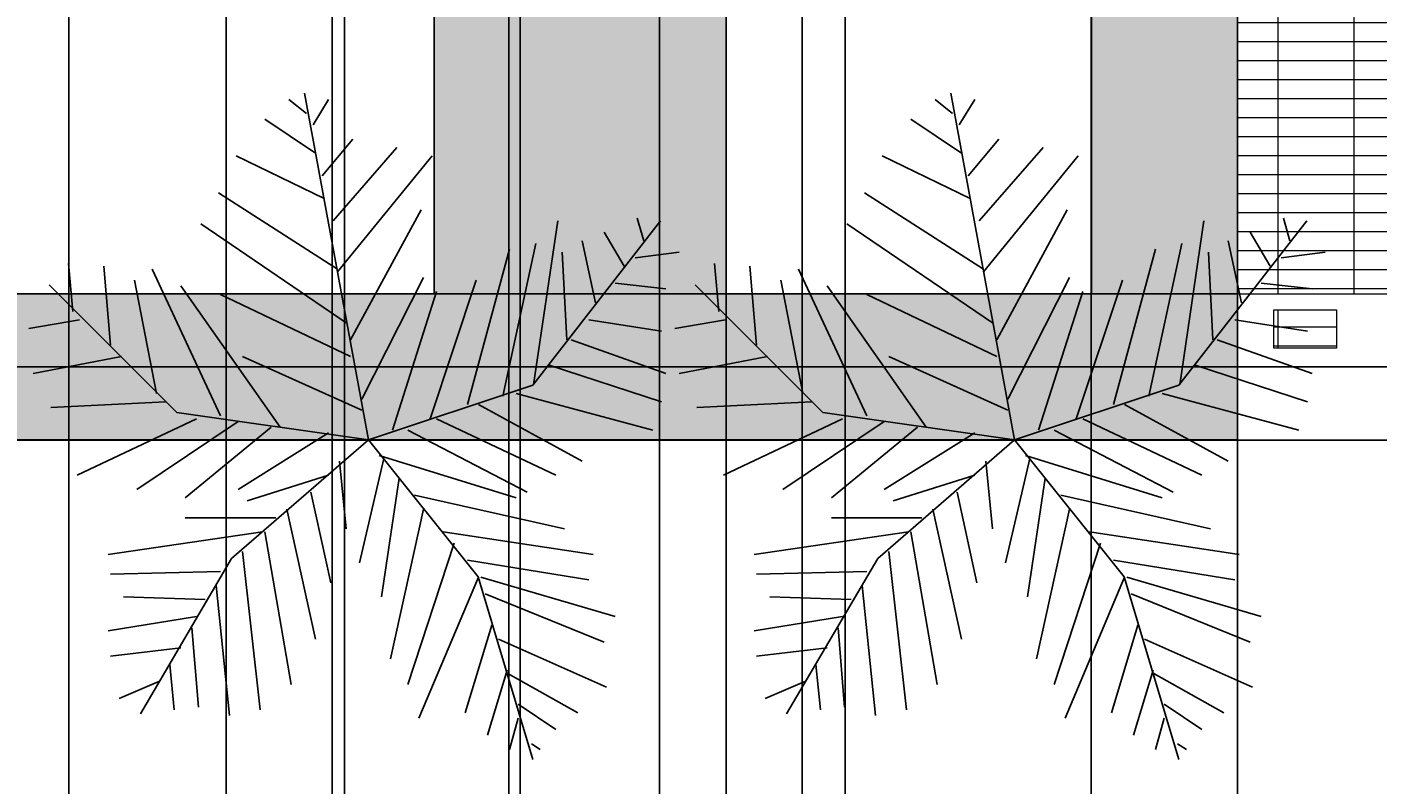
# Model space of a CAD drawing. Units: inches. Extents: x 484 to 1264, y 95 to 991.
# Tile 3 of 8: x 657 to 879, y 250 to 374. Entities that reach past the tile are written whole.
import ezdxf

# ---------------------------------------------------------------- set-up
doc = ezdxf.new("R2010")
doc.units = ezdxf.units.IN
doc.header["$MEASUREMENT"] = 0
for name, color, linetype, lineweight in [('A-ANNO-DIMS', 2, 'Continuous', 18), ('L-FENC', 7, 'Continuous', 25), ('L-FENC-GRIL-PATT', 6, 'Continuous', 13), ('L-GATE', 7, 'Continuous', 18)]:
    doc.layers.add(name, color=color, linetype=linetype, lineweight=lineweight)
doc.layers.add('L-FENC-PATT', color=34, linetype='Continuous', lineweight=13, true_color=0xa25420)
doc.layers.add('TREES', color=92, linetype='Continuous')
doc.styles.get("Standard").update_dxf_attribs({"font": 'arial.ttf'})
doc.dimstyles.get("Standard").update_dxf_attribs({"dimtxt": 0.18, "dimasz": 0.18, "dimexe": 0.18, "dimexo": 0.0625, "dimgap": 0.09, "dimtad": 0, "dimtih": 1, "dimtoh": 1, "dimdec": 4, "dimzin": 0, "dimdsep": 46, "dimtxsty": 'Standard', "dimcen": 0.09, "dimadec": 0, "dimazin": 0, "dimtfac": 1, "dimtdec": 4, "dimtofl": 0, "dimtmove": 0, "dimatfit": 3, "dimfxl": 1, "dimtolj": 1, "dimtzin": 0, "dimarcsym": 0})

# ---------------------------------------------------------------- blocks, each defined once
blk = doc.blocks.new('*U2')
for p, q in [((-10.186, 53.64), (-13.084, 55.962)), ((0, 0), (-10.5, 57)), ((-9.099, 51.782), (-6.563, 55.962)), ((-8.737, 47.138), (-17.069, 52.711)), ((-7.65, 43.423), (-2.578, 49.46)), ((-7.288, 39.707), (-21.778, 46.673)), ((-5.839, 35.992), (4.667, 48.067)), ((-5.114, 27.632), (10.463, 46.673)), ((-5.114, 28.097), (-24.676, 40.636)), ((-2.941, 16.486), (8.652, 37.85)), ((-3.665, 19.273), (-27.574, 35.527)), ((27, 9), (48, 36)), ((27.127, 9.056), (31.112, 35.992)), ((44.153, 36.456), (45.239, 32.741)), ((38.719, 34.134), (41.979, 28.561)), ((16.259, 5.805), (23.142, 31.348)), ((22.055, 7.198), (27.489, 32.277)), ((35.096, 32.741), (37.27, 22.524)), ((-48.585, 21.131), (-49.309, 29.026)), ((31.836, 30.883), (32.561, 16.486)), ((43.791, 29.954), (51.036, 30.883)), ((-43.513, 28.561), (-42.427, 15.558)), ((-35.544, 28.097), (-24.314, 3.947)), ((-1.129, 6.734), (9.014, 26.704)), ((-31.5, 4.5), (-52.5, 25.5)), ((-38.442, 26.239), (-34.819, 7.663)), ((-14.533, 2.09), (-30.834, 25.31)), ((10.101, 3.483), (17.708, 26.239)), ((40.53, 25.775), (48.862, 24.846)), ((-24.314, 23.917), (-2.941, 13.7)), ((3.942, 1.625), (11.187, 24.381)), ((-47.498, 19.737), (-55.83, 18.344)), ((36.183, 19.737), (48.137, 17.88)), ((33.285, 16.486), (48.862, 10.913)), ((-40.615, 13.7), (-55.105, 10.913)), ((-20.691, 13.7), (-1.129, 4.876)), ((29.662, 12.307), (48.137, 6.269)), ((0, 0), (27, 9)), ((24.229, 7.663), (46.688, 1.625)), ((-33.37, 6.269), (-52.207, 5.34)), ((0, 0), (-31.5, 4.5)), ((18.07, 5.805), (35.096, -3.483)), ((-28.299, 3.483), (-47.86, -5.805)), ((-21.416, 3.018), (-38.079, -8.128)), ((11.187, 3.483), (30.749, -5.805)), ((-15.982, 2.09), (-30.11, -9.521)), ((0, 0), (-22.5, -19.5)), ((-6.563, 1.161), (-21.416, -8.128)), ((0, 0), (18, -22.5)), ((6.478, 1.625), (26.04, -8.592)), ((-4.752, -3.483), (-3.665, -14.629)), ((2.493, -3.019), (-1.491, -20.202)), ((1.769, -2.555), (24.229, -9.521)), ((-6.563, -5.805), (-19.967, -9.985)), ((5.029, -6.27), (2.131, -25.775)), ((-9.461, -8.592), (-6.201, -23.453)), ((7.565, -9.056), (32.198, -14.629)), ((-15.257, -12.772), (-30.11, -12.772)), ((-13.446, -11.378), (-8.737, -32.741)), ((9.014, -11.378), (3.58, -35.992)), ((-17.431, -15.094), (-42.789, -18.809)), ((-17.069, -15.094), (-12.721, -40.172)), ((12.274, -15.094), (36.907, -18.809)), ((14.085, -16.951), (6.478, -40.172)), ((-22.5, -19.5), (-37.5, -45)), ((-20.691, -18.345), (-17.793, -44.352)), ((16.259, -19.738), (36.183, -22.989)), ((-24.314, -21.596), (-42.427, -22.06)), ((-25.038, -23.918), (-22.865, -45.281)), ((18.07, -22.524), (8.289, -45.745)), ((18, -22.5), (27, -52.5)), ((18.433, -22.524), (40.53, -29.026)), ((-26.849, -26.24), (-40.253, -25.775)), ((19.157, -25.311), (38.719, -33.206)), ((-28.299, -29.026), (-42.789, -31.348)), ((-29.023, -30.884), (-27.936, -43.887)), ((20.244, -30.419), (15.897, -44.816)), ((21.331, -32.741), (39.081, -40.636)), ((-30.834, -34.135), (-42.427, -35.528)), ((-32.646, -36.921), (-31.921, -44.352)), ((-34.457, -39.708), (-40.978, -42.494)), ((22.78, -37.85), (19.519, -48.532)), ((22.78, -38.314), (34.372, -44.816)), ((24.591, -43.423), (30.749, -47.603)), ((24.591, -45.745), (23.142, -50.854)), ((26.764, -49.925), (28.213, -50.854))]:
    blk.add_line(p, q)
blk = doc.blocks.new('GATE-LOWER-INSET')
blk.add_lwpolyline([(0, 6.26), (10.31, 6.26), (10.31, 0), (0, 0)], close=True)
blk = doc.blocks.new('*D16')
at = {"layer": 'A-ANNO-DIMS', "color": 0, "lineweight": -2, "transparency": 16777216}
for p, q in [((639.81, 408.32), (639.81, 94.79)), ((999.81, 318.32), (999.81, 94.79)), ((639.99, 94.97), (819.53, 94.97)), ((999.63, 94.97), (820.1, 94.97))]:
    blk.add_line(p, q, dxfattribs=at)
at = {"layer": 'A-ANNO-DIMS', "color": 0, "transparency": 16777216}
for points in [[(639.99, 95), (639.99, 94.94), (639.81, 94.97)], [(999.63, 95), (999.63, 94.94), (999.81, 94.97)]]:
    blk.add_solid(points, dxfattribs=at)
at = {"layer": 'Defpoints', "color": 0, "transparency": 16777216}
for p in [(639.81, 408.38), (999.81, 318.38), (999.81, 94.97)]:
    blk.add_point(p, dxfattribs=at)
at = {"layer": 'A-ANNO-DIMS', "color": 0, "transparency": 16777216, "insert": (819.81, 94.97), "char_height": 0.18, "attachment_point": 5}
blk.add_mtext('\\A1;360', dxfattribs=at)
blk = doc.blocks.new('*D17')
at = {"layer": 'A-ANNO-DIMS', "color": 0, "lineweight": -2, "transparency": 16777216}
for p, q in [((709.01, 950.08), (484.15, 950.08)), ((484.33, 949.9), (484.33, 628.41)), ((484.33, 306.56), (484.33, 628.05)), ((595.26, 306.38), (484.15, 306.38))]:
    blk.add_line(p, q, dxfattribs=at)
at = {"layer": 'A-ANNO-DIMS', "color": 0, "transparency": 16777216}
for points in [[(484.3, 949.9), (484.36, 949.9), (484.33, 950.08)], [(484.3, 306.56), (484.36, 306.56), (484.33, 306.38)]]:
    blk.add_solid(points, dxfattribs=at)
at = {"layer": 'Defpoints', "color": 0, "transparency": 16777216}
for p in [(484.33, 950.08), (709.07, 950.08), (595.32, 306.38)]:
    blk.add_point(p, dxfattribs=at)
at = {"layer": 'A-ANNO-DIMS', "color": 0, "transparency": 16777216, "insert": (484.33, 628.23), "char_height": 0.18, "attachment_point": 5}
blk.add_mtext('\\A1;643.7', dxfattribs=at)
blk = doc.blocks.new('*D18')
at = {"layer": 'A-ANNO-DIMS', "color": 0, "lineweight": -2, "transparency": 16777216}
for p, q in [((999.88, 501.38), (1264.08, 501.38)), ((1263.9, 501.2), (1263.9, 404.07)), ((1263.9, 306.56), (1263.9, 403.7)), ((595.38, 306.38), (1264.08, 306.38))]:
    blk.add_line(p, q, dxfattribs=at)
at = {"layer": 'A-ANNO-DIMS', "color": 0, "transparency": 16777216}
for points in [[(1263.87, 501.2), (1263.93, 501.2), (1263.9, 501.38)], [(1263.87, 306.56), (1263.93, 306.56), (1263.9, 306.38)]]:
    blk.add_solid(points, dxfattribs=at)
at = {"layer": 'Defpoints', "color": 0, "transparency": 16777216}
for p in [(999.81, 501.38), (1263.9, 501.38), (595.32, 306.38)]:
    blk.add_point(p, dxfattribs=at)
at = {"layer": 'A-ANNO-DIMS', "color": 0, "transparency": 16777216, "insert": (1263.9, 403.88), "char_height": 0.18, "attachment_point": 5}
blk.add_mtext('\\A1;195', dxfattribs=at)
blk = doc.blocks.new('*D23')
at = {"layer": 'A-ANNO-DIMS', "color": 0, "lineweight": -2, "transparency": 16777216}
for p, q in [((663.81, 906.32), (663.81, 94.79)), ((709.07, 889.06), (709.07, 94.79)), ((663.99, 94.97), (686.04, 94.97)), ((708.89, 94.97), (686.84, 94.97))]:
    blk.add_line(p, q, dxfattribs=at)
at = {"layer": 'A-ANNO-DIMS', "color": 0, "transparency": 16777216}
for points in [[(663.99, 95), (663.99, 94.94), (663.81, 94.97)], [(708.89, 95), (708.89, 94.94), (709.07, 94.97)]]:
    blk.add_solid(points, dxfattribs=at)
at = {"layer": 'Defpoints', "color": 0, "transparency": 16777216}
for p in [(663.81, 906.38), (709.07, 889.12), (709.07, 94.97)]:
    blk.add_point(p, dxfattribs=at)
at = {"layer": 'A-ANNO-DIMS', "color": 0, "transparency": 16777216, "insert": (686.44, 94.97), "char_height": 0.18, "attachment_point": 5}
blk.add_mtext('\\A1;45.25', dxfattribs=at)
blk = doc.blocks.new('*D24')
at = {"layer": 'A-ANNO-DIMS', "color": 0, "lineweight": -2, "transparency": 16777216}
for p, q in [((709.07, 889.06), (709.07, 94.79)), ((736.12, 889.06), (736.12, 94.79)), ((709.25, 94.97), (722.2, 94.97)), ((735.94, 94.97), (722.99, 94.97))]:
    blk.add_line(p, q, dxfattribs=at)
at = {"layer": 'A-ANNO-DIMS', "color": 0, "transparency": 16777216}
for points in [[(709.25, 95), (709.25, 94.94), (709.07, 94.97)], [(735.94, 95), (735.94, 94.94), (736.12, 94.97)]]:
    blk.add_solid(points, dxfattribs=at)
at = {"layer": 'Defpoints', "color": 0, "transparency": 16777216}
for p in [(709.07, 889.12), (736.12, 889.12), (736.12, 94.97)]:
    blk.add_point(p, dxfattribs=at)
at = {"layer": 'A-ANNO-DIMS', "color": 0, "transparency": 16777216, "insert": (722.59, 94.97), "char_height": 0.18, "attachment_point": 5}
blk.add_mtext('\\A1;27.05', dxfattribs=at)
blk = doc.blocks.new('*D25')
at = {"layer": 'A-ANNO-DIMS', "color": 0, "lineweight": -2, "transparency": 16777216}
for p, q in [((736.12, 889.06), (736.12, 94.79)), ((760.87, 889.06), (760.87, 94.79)), ((736.3, 94.97), (748.1, 94.97)), ((760.69, 94.97), (748.89, 94.97))]:
    blk.add_line(p, q, dxfattribs=at)
at = {"layer": 'A-ANNO-DIMS', "color": 0, "transparency": 16777216}
for points in [[(736.3, 95), (736.3, 94.94), (736.12, 94.97)], [(760.69, 95), (760.69, 94.94), (760.87, 94.97)]]:
    blk.add_solid(points, dxfattribs=at)
at = {"layer": 'Defpoints', "color": 0, "transparency": 16777216}
for p in [(736.12, 889.12), (760.87, 889.12), (760.87, 94.97)]:
    blk.add_point(p, dxfattribs=at)
at = {"layer": 'A-ANNO-DIMS', "color": 0, "transparency": 16777216, "insert": (748.49, 94.97), "char_height": 0.18, "attachment_point": 5}
blk.add_mtext('\\A1;24.75', dxfattribs=at)
blk = doc.blocks.new('*D26')
at = {"layer": 'A-ANNO-DIMS', "color": 0, "lineweight": -2, "transparency": 16777216}
for p, q in [((689.66, 819.99), (689.66, 94.79)), ((663.81, 810.32), (663.81, 94.79)), ((663.99, 94.97), (676.27, 94.97)), ((689.48, 94.97), (677.2, 94.97))]:
    blk.add_line(p, q, dxfattribs=at)
at = {"layer": 'A-ANNO-DIMS', "color": 0, "transparency": 16777216}
for points in [[(663.99, 95), (663.99, 94.94), (663.81, 94.97)], [(689.48, 95), (689.48, 94.94), (689.66, 94.97)]]:
    blk.add_solid(points, dxfattribs=at)
at = {"layer": 'Defpoints', "color": 0, "transparency": 16777216}
for p in [(689.66, 820.06), (663.81, 810.38), (689.66, 94.97)]:
    blk.add_point(p, dxfattribs=at)
at = {"layer": 'A-ANNO-DIMS', "color": 0, "transparency": 16777216, "insert": (676.74, 94.97), "char_height": 0.18, "attachment_point": 5}
blk.add_mtext('\\A1;25.846', dxfattribs=at)
blk = doc.blocks.new('*D27')
at = {"layer": 'A-ANNO-DIMS', "color": 0, "lineweight": -2, "transparency": 16777216}
for p, q in [((689.66, 819.99), (689.66, 94.79)), ((737.98, 819.99), (737.98, 94.79)), ((689.84, 94.97), (713.42, 94.97)), ((737.8, 94.97), (714.22, 94.97))]:
    blk.add_line(p, q, dxfattribs=at)
at = {"layer": 'A-ANNO-DIMS', "color": 0, "transparency": 16777216}
for points in [[(689.84, 95), (689.84, 94.94), (689.66, 94.97)], [(737.8, 95), (737.8, 94.94), (737.98, 94.97)]]:
    blk.add_solid(points, dxfattribs=at)
at = {"layer": 'Defpoints', "color": 0, "transparency": 16777216}
for p in [(689.66, 820.06), (737.98, 820.06), (737.98, 94.97)]:
    blk.add_point(p, dxfattribs=at)
at = {"layer": 'A-ANNO-DIMS', "color": 0, "transparency": 16777216, "insert": (713.82, 94.97), "char_height": 0.18, "attachment_point": 5}
blk.add_mtext('\\A1;48.32', dxfattribs=at)
blk = doc.blocks.new('*D28')
at = {"layer": 'A-ANNO-DIMS', "color": 0, "lineweight": -2, "transparency": 16777216}
for p, q in [((737.98, 819.99), (737.98, 94.79)), ((784.3, 819.99), (784.3, 94.79)), ((738.16, 94.97), (760.67, 94.97)), ((784.12, 94.97), (761.61, 94.97))]:
    blk.add_line(p, q, dxfattribs=at)
at = {"layer": 'A-ANNO-DIMS', "color": 0, "transparency": 16777216}
for points in [[(738.16, 95), (738.16, 94.94), (737.98, 94.97)], [(784.12, 95), (784.12, 94.94), (784.3, 94.97)]]:
    blk.add_solid(points, dxfattribs=at)
at = {"layer": 'Defpoints', "color": 0, "transparency": 16777216}
for p in [(737.98, 820.06), (784.3, 820.06), (784.3, 94.97)]:
    blk.add_point(p, dxfattribs=at)
at = {"layer": 'A-ANNO-DIMS', "color": 0, "transparency": 16777216, "insert": (761.14, 94.97), "char_height": 0.18, "attachment_point": 5}
blk.add_mtext('\\A1;46.325', dxfattribs=at)
blk = doc.blocks.new('*D29')
at = {"layer": 'A-ANNO-DIMS', "color": 0, "lineweight": -2, "transparency": 16777216}
for p, q in [((831.81, 906.32), (831.81, 94.79)), ((784.3, 819.99), (784.3, 94.79)), ((784.48, 94.97), (807.68, 94.97)), ((831.63, 94.97), (808.44, 94.97))]:
    blk.add_line(p, q, dxfattribs=at)
at = {"layer": 'A-ANNO-DIMS', "color": 0, "transparency": 16777216}
for points in [[(784.48, 95), (784.48, 94.94), (784.3, 94.97)], [(831.63, 95), (831.63, 94.94), (831.81, 94.97)]]:
    blk.add_solid(points, dxfattribs=at)
at = {"layer": 'Defpoints', "color": 0, "transparency": 16777216}
for p in [(831.81, 906.38), (784.3, 820.06), (831.81, 94.97)]:
    blk.add_point(p, dxfattribs=at)
at = {"layer": 'A-ANNO-DIMS', "color": 0, "transparency": 16777216, "insert": (808.06, 94.97), "char_height": 0.18, "attachment_point": 5}
blk.add_mtext('\\A1;47.51', dxfattribs=at)
blk = doc.blocks.new('*D33')
at = {"layer": 'A-ANNO-DIMS', "color": 0, "lineweight": -2, "transparency": 16777216}
for p, q in [((639.81, 930.32), (639.81, 94.79)), ((663.81, 810.32), (663.81, 94.79)), ((639.99, 94.97), (651.59, 94.97)), ((663.63, 94.97), (652.03, 94.97))]:
    blk.add_line(p, q, dxfattribs=at)
at = {"layer": 'A-ANNO-DIMS', "color": 0, "transparency": 16777216}
for points in [[(639.99, 95), (639.99, 94.94), (639.81, 94.97)], [(663.63, 95), (663.63, 94.94), (663.81, 94.97)]]:
    blk.add_solid(points, dxfattribs=at)
at = {"layer": 'Defpoints', "color": 0, "transparency": 16777216}
for p in [(639.81, 930.38), (663.81, 810.38), (663.81, 94.97)]:
    blk.add_point(p, dxfattribs=at)
at = {"layer": 'A-ANNO-DIMS', "color": 0, "transparency": 16777216, "insert": (651.81, 94.97), "char_height": 0.18, "attachment_point": 5}
blk.add_mtext('\\A1;24', dxfattribs=at)
blk = doc.blocks.new('*D36')
at = {"layer": 'A-ANNO-DIMS', "color": 0, "lineweight": -2, "transparency": 16777216}
for p, q in [((707.04, 581.21), (707.04, 94.79)), ((663.81, 501.32), (663.81, 94.79)), ((663.99, 94.97), (685.03, 94.97)), ((706.86, 94.97), (685.82, 94.97))]:
    blk.add_line(p, q, dxfattribs=at)
at = {"layer": 'A-ANNO-DIMS', "color": 0, "transparency": 16777216}
for points in [[(663.99, 95), (663.99, 94.94), (663.81, 94.97)], [(706.86, 95), (706.86, 94.94), (707.04, 94.97)]]:
    blk.add_solid(points, dxfattribs=at)
at = {"layer": 'Defpoints', "color": 0, "transparency": 16777216}
for p in [(707.04, 581.28), (663.81, 501.38), (707.04, 94.97)]:
    blk.add_point(p, dxfattribs=at)
at = {"layer": 'A-ANNO-DIMS', "color": 0, "transparency": 16777216, "insert": (685.43, 94.97), "char_height": 0.18, "attachment_point": 5}
blk.add_mtext('\\A1;43.22', dxfattribs=at)
blk = doc.blocks.new('*D37')
at = {"layer": 'A-ANNO-DIMS', "color": 0, "lineweight": -2, "transparency": 16777216}
for p, q in [((707.04, 581.21), (707.04, 94.79)), ((791.36, 581.21), (791.36, 94.79)), ((707.22, 94.97), (748.81, 94.97)), ((791.18, 94.97), (749.59, 94.97))]:
    blk.add_line(p, q, dxfattribs=at)
at = {"layer": 'A-ANNO-DIMS', "color": 0, "transparency": 16777216}
for points in [[(707.22, 95), (707.22, 94.94), (707.04, 94.97)], [(791.18, 95), (791.18, 94.94), (791.36, 94.97)]]:
    blk.add_solid(points, dxfattribs=at)
at = {"layer": 'Defpoints', "color": 0, "transparency": 16777216}
for p in [(707.04, 581.28), (791.36, 581.28), (791.36, 94.97)]:
    blk.add_point(p, dxfattribs=at)
at = {"layer": 'A-ANNO-DIMS', "color": 0, "transparency": 16777216, "insert": (749.2, 94.97), "char_height": 0.18, "attachment_point": 5}
blk.add_mtext('\\A1;84.32', dxfattribs=at)
blk = doc.blocks.new('*D49')
at = {"layer": 'A-ANNO-DIMS', "color": 0, "lineweight": -2, "transparency": 16777216}
for p, q in [((855.81, 318.32), (855.81, 94.79)), ((975.81, 318.32), (975.81, 94.79)), ((855.99, 94.97), (915.53, 94.97)), ((975.63, 94.97), (916.09, 94.97))]:
    blk.add_line(p, q, dxfattribs=at)
at = {"layer": 'A-ANNO-DIMS', "color": 0, "transparency": 16777216}
for points in [[(855.99, 95), (855.99, 94.94), (855.81, 94.97)], [(975.63, 95), (975.63, 94.94), (975.81, 94.97)]]:
    blk.add_solid(points, dxfattribs=at)
at = {"layer": 'Defpoints', "color": 0, "transparency": 16777216}
for p in [(855.81, 318.38), (975.81, 318.38), (975.81, 94.97)]:
    blk.add_point(p, dxfattribs=at)
at = {"layer": 'A-ANNO-DIMS', "color": 0, "transparency": 16777216, "insert": (915.81, 94.97), "char_height": 0.18, "attachment_point": 5}
blk.add_mtext('\\A1;120', dxfattribs=at)
blk = doc.blocks.new('*D51')
at = {"layer": 'A-ANNO-DIMS', "color": 0, "lineweight": -2, "transparency": 16777216}
for p, q in [((869.55, 421.47), (484.15, 421.47)), ((484.33, 421.29), (484.33, 370.11)), ((484.33, 318.56), (484.33, 369.75)), ((855.75, 318.38), (484.15, 318.38))]:
    blk.add_line(p, q, dxfattribs=at)
at = {"layer": 'A-ANNO-DIMS', "color": 0, "transparency": 16777216}
for points in [[(484.3, 421.29), (484.36, 421.29), (484.33, 421.47)], [(484.3, 318.56), (484.36, 318.56), (484.33, 318.38)]]:
    blk.add_solid(points, dxfattribs=at)
at = {"layer": 'Defpoints', "color": 0, "transparency": 16777216}
for p in [(484.33, 421.47), (869.61, 421.47), (855.81, 318.38)]:
    blk.add_point(p, dxfattribs=at)
at = {"layer": 'A-ANNO-DIMS', "color": 0, "transparency": 16777216, "insert": (484.33, 369.93), "char_height": 0.18, "attachment_point": 5}
blk.add_mtext('\\A1;103.09', dxfattribs=at)
blk = doc.blocks.new('*D53')
at = {"layer": 'A-ANNO-DIMS', "color": 0, "lineweight": -2, "transparency": 16777216}
for p, q in [((771.81, 330.32), (771.81, 94.79)), ((831.81, 330.32), (831.81, 94.79)), ((771.99, 94.97), (801.6, 94.97)), ((831.63, 94.97), (802.03, 94.97))]:
    blk.add_line(p, q, dxfattribs=at)
at = {"layer": 'A-ANNO-DIMS', "color": 0, "transparency": 16777216}
for points in [[(771.99, 95), (771.99, 94.94), (771.81, 94.97)], [(831.63, 95), (831.63, 94.94), (831.81, 94.97)]]:
    blk.add_solid(points, dxfattribs=at)
at = {"layer": 'Defpoints', "color": 0, "transparency": 16777216}
for p in [(771.81, 330.38), (831.81, 330.38), (831.81, 94.97)]:
    blk.add_point(p, dxfattribs=at)
at = {"layer": 'A-ANNO-DIMS', "color": 0, "transparency": 16777216, "insert": (801.81, 94.97), "char_height": 0.18, "attachment_point": 5}
blk.add_mtext('\\A1;60', dxfattribs=at)
blk = doc.blocks.new('*D58')
at = {"layer": 'A-ANNO-DIMS', "color": 0, "lineweight": -2, "transparency": 16777216}
for p, q in [((855.75, 396.38), (484.15, 396.38)), ((484.33, 396.2), (484.33, 363.57)), ((484.33, 330.56), (484.33, 363.2)), ((855.75, 330.38), (484.15, 330.38))]:
    blk.add_line(p, q, dxfattribs=at)
at = {"layer": 'A-ANNO-DIMS', "color": 0, "transparency": 16777216}
for points in [[(484.3, 396.2), (484.36, 396.2), (484.33, 396.38)], [(484.3, 330.56), (484.36, 330.56), (484.33, 330.38)]]:
    blk.add_solid(points, dxfattribs=at)
at = {"layer": 'Defpoints', "color": 0, "transparency": 16777216}
for p in [(484.33, 396.38), (855.81, 396.38), (855.81, 330.38)]:
    blk.add_point(p, dxfattribs=at)
at = {"layer": 'A-ANNO-DIMS', "color": 0, "transparency": 16777216, "insert": (484.33, 363.38), "char_height": 0.18, "attachment_point": 5}
blk.add_mtext('\\A1;66', dxfattribs=at)
blk = doc.blocks.new('*D59')
at = {"layer": 'A-ANNO-DIMS', "color": 0, "lineweight": -2, "transparency": 16777216}
for p, q in [((855.88, 318.38), (1264.08, 318.38)), ((1263.9, 318.2), (1263.9, 312.56)), ((1263.9, 306.56), (1263.9, 312.2)), ((855.88, 306.38), (1264.08, 306.38))]:
    blk.add_line(p, q, dxfattribs=at)
at = {"layer": 'A-ANNO-DIMS', "color": 0, "transparency": 16777216}
for points in [[(1263.87, 318.2), (1263.93, 318.2), (1263.9, 318.38)], [(1263.87, 306.56), (1263.93, 306.56), (1263.9, 306.38)]]:
    blk.add_solid(points, dxfattribs=at)
at = {"layer": 'Defpoints', "color": 0, "transparency": 16777216}
for p in [(855.81, 318.38), (855.81, 306.38), (1263.9, 306.38)]:
    blk.add_point(p, dxfattribs=at)
at = {"layer": 'A-ANNO-DIMS', "color": 0, "transparency": 16777216, "insert": (1263.9, 312.38), "char_height": 0.18, "attachment_point": 5}
blk.add_mtext('\\A1;12', dxfattribs=at)
blk = doc.blocks.new('*D60')
at = {"layer": 'A-ANNO-DIMS', "color": 0, "lineweight": -2, "transparency": 16777216}
for p, q in [((855.75, 330.38), (484.15, 330.38)), ((484.33, 330.2), (484.33, 324.56)), ((484.33, 318.56), (484.33, 324.2)), ((855.75, 318.38), (484.15, 318.38))]:
    blk.add_line(p, q, dxfattribs=at)
at = {"layer": 'A-ANNO-DIMS', "color": 0, "transparency": 16777216}
for points in [[(484.3, 330.2), (484.36, 330.2), (484.33, 330.38)], [(484.3, 318.56), (484.36, 318.56), (484.33, 318.38)]]:
    blk.add_solid(points, dxfattribs=at)
at = {"layer": 'Defpoints', "color": 0, "transparency": 16777216}
for p in [(484.33, 330.38), (855.81, 330.38), (855.81, 318.38)]:
    blk.add_point(p, dxfattribs=at)
at = {"layer": 'A-ANNO-DIMS', "color": 0, "transparency": 16777216, "insert": (484.33, 324.38), "char_height": 0.18, "attachment_point": 5}
blk.add_mtext('\\A1;12', dxfattribs=at)

msp = doc.modelspace()

# ---------------------------------------------------------------- hatches: boundary and pattern name
at = {"layer": 'L-FENC-GRIL-PATT'}
h = msp.add_hatch(dxfattribs=at)
h.set_pattern_fill('GRATE', color=256, scale=100)
h.paths.add_polyline_path([(974.8147, 396.3846), (927.8147, 396.3846), (927.8147, 330.3846), (974.8147, 330.3846)])
h.paths.add_polyline_path([(903.8147, 396.3846), (855.8147, 396.3846), (855.8147, 330.3846), (903.8147, 330.3846)])
h.paths.add_polyline_path([(819.8147, 420.3846), (807.8147, 420.3846), (807.8147, 408.3846), (819.8147, 408.3846)])
h.paths.add_polyline_path([(807.8147, 420.3846), (795.8147, 420.3846), (795.8147, 408.3846), (807.8147, 408.3846)])
h.paths.add_polyline_path([(795.8147, 420.3846), (783.8147, 420.3846), (783.8147, 408.3846), (795.8147, 408.3846)])
h.paths.add_polyline_path([(831.8147, 420.3846), (819.8147, 420.3846), (819.8147, 408.3846), (831.8147, 408.3846)])
h.paths.add_polyline_path([(783.8147, 420.3846), (779.9105, 420.3846), (779.9105, 412.138), (771.8147, 412.138), (771.8147, 408.3846), (783.8147, 408.3846)])
h.paths.add_polyline_path([(777.9105, 420.3846), (771.8147, 420.3846), (771.8147, 414.138), (777.9105, 414.138)], flags=17)
h.paths.add_polyline_path([(723.8147, 420.3846), (711.8147, 420.3846), (711.8147, 408.3846), (723.8147, 408.3846)])
h.paths.add_polyline_path([(711.8147, 420.3846), (699.8147, 420.3846), (699.8147, 408.3846), (711.8147, 408.3846)])
h.paths.add_polyline_path([(699.8147, 420.3846), (687.8147, 420.3846), (687.8147, 408.3846), (699.8147, 408.3846)])
h.paths.add_polyline_path([(687.8147, 420.3846), (675.8147, 420.3846), (675.8147, 408.3846), (687.8147, 408.3846)])
h.paths.add_polyline_path([(675.8147, 420.3846), (663.8147, 420.3846), (663.8147, 408.3846), (675.8147, 408.3846)])
h.paths.add_polyline_path([(639.8147, 420.3846), (631.3221, 420.3846), (631.3221, 408.3846), (639.8147, 408.3846)])
h.paths.add_polyline_path([(631.3221, 420.3846), (619.3221, 420.3846), (619.3221, 408.3846), (631.3221, 408.3846)])
h = msp.add_hatch(dxfattribs=at)
h.set_pattern_fill('GRATE', color=256, scale=100)
h.paths.add_polyline_path([(965.5846, 327.7657), (955.27, 327.7657), (955.27, 321.5012), (965.5846, 321.5012)])
h.paths.add_polyline_path([(943.7309, 327.7657), (933.4163, 327.7657), (933.4163, 321.5012), (943.7309, 321.5012)])
h.paths.add_polyline_path([(893.9522, 327.7657), (883.6376, 327.7657), (883.6376, 321.5012), (893.9522, 321.5012)])
h.paths.add_polyline_path([(872.1278, 327.7657), (861.8132, 327.7657), (861.8132, 321.5012), (872.1278, 321.5012)])
at = {"layer": 'L-FENC-PATT'}
h = msp.add_hatch(color=256, dxfattribs=at)
h.dxf.hatch_style = 1
h.paths.add_polyline_path([(619.3221, 420.3846), (595.3221, 420.3846), (595.3221, 306.3846), (855.8147, 306.3846), (855.8147, 420.3846), (831.8147, 420.3846), (831.8147, 330.3846), (771.8147, 330.3846), (771.8147, 420.3846), (723.8147, 420.3846), (723.8147, 330.3846), (619.3221, 330.3846)])
h.paths.add_polyline_path([(999.8147, 420.3846), (975.8147, 420.3846), (975.8147, 318.3846), (999.8147, 318.3846)])

# ---------------------------------------------------------------- linework, layer by layer
at = {"layer": 'L-FENC'}
for p, q in [((723.8147, 420.3846), (723.8147, 330.3846)), ((771.8147, 420.3846), (771.8147, 330.3846)), ((831.8147, 420.4387), (831.8147, 330.3846)), ((855.8147, 420.3846), (855.8147, 306.3846)), ((619.3221, 330.3846), (723.8147, 330.3846)), ((771.8147, 330.3846), (831.8147, 330.3846)), ((595.3221, 306.3846), (855.8147, 306.3846))]:
    msp.add_line(p, q, dxfattribs=at)
at = {"layer": 'L-GATE'}
for p, q in [((855.8147, 330.3846), (903.8147, 330.3846)), ((855.8147, 318.3846), (999.8147, 318.3846))]:
    msp.add_line(p, q, dxfattribs=at)

# ---------------------------------------------------------------- block references
msp.add_blockref('GATE-LOWER-INSET', (861.8132, 321.5012), dxfattribs=at)
at = {"layer": 'TREES'}
for p in [(713.044, 306.3846), (819.2113, 306.3846)]:
    msp.add_blockref('*U2', p, dxfattribs=at)

# ---------------------------------------------------------------- dimensions: what is measured, and where the dimension line sits
at = {"layer": 'A-ANNO-DIMS'}
for base, p1, p2, override, picture, middle in [((484.3261, 950.079), (595.3221, 306.3846), (709.0683, 950.079), {"dimdec": 1, "dimlfac": 1, "dimrnd": 0, "dimzin": 0, "dimdsep": 46, "dimlunit": 2}, '*D17', (484.3261, 628.2318)), ((1263.9032, 501.3846), (595.3221, 306.3846), (999.8147, 501.3846), {"dimdec": 0, "dimlfac": 1, "dimrnd": 0, "dimzin": 0, "dimdsep": 46, "dimlunit": 2}, '*D18', (1263.9032, 403.8846)), ((484.3261, 421.4725), (855.8147, 318.3846), (869.6148, 421.4725), {"dimdec": 2, "dimlfac": 1, "dimrnd": 0, "dimzin": 0, "dimdsep": 46, "dimlunit": 2}, '*D51', (484.3261, 369.9286)), ((484.3261, 396.3846), (855.8147, 330.3846), (855.8147, 396.3846), {"dimdec": 0, "dimlfac": 1, "dimrnd": 0, "dimzin": 0, "dimdsep": 46, "dimlunit": 2}, '*D58', (484.3261, 363.3846)), ((484.3261, 330.3846), (855.8147, 318.3846), (855.8147, 330.3846), {"dimdec": 0, "dimlfac": 1, "dimrnd": 0, "dimzin": 0, "dimdsep": 46, "dimlunit": 2}, '*D60', (484.3261, 324.3846)), ((1263.9032, 306.3846), (855.8147, 318.3846), (855.8147, 306.3846), {"dimdec": 0, "dimlfac": 1, "dimrnd": 0, "dimzin": 0, "dimdsep": 46, "dimlunit": 2}, '*D59', (1263.9032, 312.3846))]:
    dim = msp.add_linear_dim(base=base, p1=p1, p2=p2, angle=90, dimstyle='Standard', override=override, dxfattribs=at)
    dim.commit()
    dim.dimension.update_dxf_attribs({"geometry": picture, "text_midpoint": middle})
for base, p1, p2, override, picture, middle in [((663.8147, 94.9714), (639.8147, 930.3846), (663.8147, 810.3846), {"dimdec": 0, "dimlfac": 1, "dimrnd": 0, "dimzin": 0, "dimdsep": 46, "dimlunit": 2}, '*D33', (651.8147, 94.9714)), ((709.0683, 94.9714), (663.8147, 906.3846), (709.0683, 889.1187), {"dimdec": 2, "dimlfac": 1, "dimrnd": 0, "dimzin": 0, "dimdsep": 46, "dimlunit": 2}, '*D23', (686.4415, 94.9714)), ((831.8147, 94.9714), (784.3024, 820.0562), (831.8147, 906.3846), {"dimdec": 2, "dimlfac": 1, "dimrnd": 0, "dimzin": 0, "dimdsep": 46, "dimlunit": 2}, '*D29', (808.0586, 94.9714)), ((736.12, 94.9714), (709.0683, 889.1187), (736.12, 889.1187), {"dimdec": 2, "dimlfac": 1, "dimrnd": 0, "dimzin": 0, "dimdsep": 46, "dimlunit": 2}, '*D24', (722.5941, 94.9714)), ((760.8695, 94.9714), (736.12, 889.1187), (760.8695, 889.1187), {"dimdec": 2, "dimlfac": 1, "dimrnd": 0, "dimzin": 0, "dimdsep": 46, "dimlunit": 2}, '*D25', (748.4947, 94.9714)), ((689.6604, 94.9714), (663.8147, 810.3846), (689.6604, 820.0562), {"dimdec": 3, "dimlfac": 1, "dimrnd": 0, "dimzin": 0, "dimdsep": 46, "dimlunit": 2}, '*D26', (676.7376, 94.9714)), ((737.9777, 94.9714), (689.6604, 820.0562), (737.9777, 820.0562), {"dimdec": 2, "dimlfac": 1, "dimrnd": 0, "dimzin": 0, "dimdsep": 46, "dimlunit": 2}, '*D27', (713.8191, 94.9714)), ((784.3024, 94.9714), (737.9777, 820.0562), (784.3024, 820.0562), {"dimdec": 3, "dimlfac": 1, "dimrnd": 0, "dimzin": 0, "dimdsep": 46, "dimlunit": 2}, '*D28', (761.1401, 94.9714)), ((707.038, 94.9714), (663.8147, 501.3846), (707.038, 581.2764), {"dimdec": 2, "dimlfac": 1, "dimrnd": 0, "dimzin": 0, "dimdsep": 46, "dimlunit": 2}, '*D36', (685.4263, 94.9714)), ((791.3605, 94.9714), (707.038, 581.2764), (791.3605, 581.2764), {"dimdec": 2, "dimlfac": 1, "dimrnd": 0, "dimzin": 0, "dimdsep": 46, "dimlunit": 2}, '*D37', (749.1992, 94.9714)), ((999.8147, 94.9714), (639.8147, 408.3846), (999.8147, 318.3846), {"dimdec": 0, "dimlfac": 1, "dimrnd": 0, "dimzin": 0, "dimdsep": 46, "dimlunit": 2}, '*D16', (819.8147, 94.9714)), ((831.8147, 94.9714), (771.8147, 330.3846), (831.8147, 330.3846), {"dimdec": 0, "dimlfac": 1, "dimrnd": 0, "dimzin": 0, "dimdsep": 46, "dimlunit": 2}, '*D53', (801.8147, 94.9714)), ((975.8147, 94.9714), (855.8147, 318.3846), (975.8147, 318.3846), {"dimdec": 0, "dimlfac": 1, "dimrnd": 0, "dimzin": 0, "dimdsep": 46, "dimlunit": 2}, '*D49', (915.8147, 94.9714))]:
    dim = msp.add_linear_dim(base=base, p1=p1, p2=p2, dimstyle='Standard', override=override, dxfattribs=at)
    dim.commit()
    dim.dimension.update_dxf_attribs({"geometry": picture, "text_midpoint": middle})

doc.saveas('drawing.dxf')
